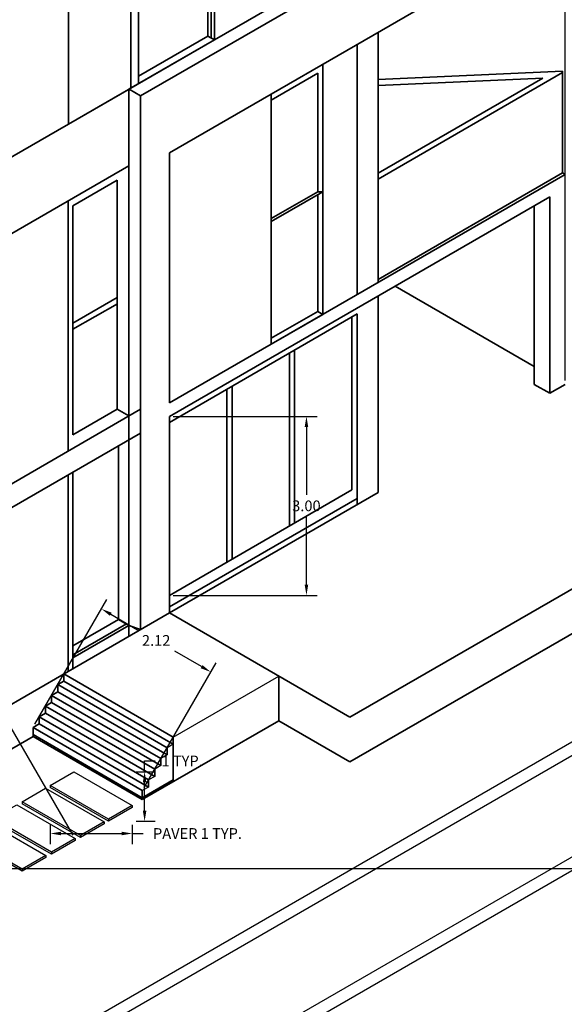
# Model space of a CAD drawing. Units: metres. Extents: x 12735 to 25554, y 20954 to 41989.
# Tile 13 of 15: x 12764 to 12773, y 20964 to 20981. Entities that reach past the tile are written whole.
import ezdxf

# ---------------------------------------------------------------- set-up
doc = ezdxf.new("R2010")
doc.units = ezdxf.units.M
doc.layers.get('Defpoints').update_dxf_attribs({"lineweight": 13})
for name, color, linetype, lineweight in [('A-ANNO-DIMS', 2, 'Continuous', 18), ('A-ELEV', 7, 'Continuous', 35), ('A-FLOR-STRS', 3, 'Continuous', 25), ('C-SITE', 8, 'Continuous', 25)]:
    doc.layers.add(name, color=color, linetype=linetype, lineweight=lineweight)
doc.styles.get("Standard").update_dxf_attribs({"font": 'arial.ttf'})
doc.dimstyles.get("Standard").update_dxf_attribs({"dimtxt": 0.18, "dimasz": 0.18, "dimexe": 0.18, "dimexo": 0.0625, "dimgap": 0.09, "dimtad": 0, "dimtih": 1, "dimtoh": 1, "dimdec": 4, "dimzin": 0, "dimdsep": 46, "dimtxsty": 'Standard', "dimcen": 0.09, "dimadec": 0, "dimazin": 0, "dimtfac": 1, "dimtdec": 4, "dimtofl": 0, "dimtmove": 0, "dimatfit": 3, "dimfxl": 1, "dimtolj": 1, "dimtzin": 0, "dimarcsym": 0})

# ---------------------------------------------------------------- blocks, each defined once
blk = doc.blocks.new('PAVER-STONE-A')
for p, q in [((0, 0.602), (0.397, 0.832)), ((0.397, 0.832), (1.377, 0.266)), ((0.98, 0.037), (0, 0.602)), ((0, 0.602), (0, 0.566)), ((0.98, 0), (0, 0.566)), ((1.377, 0.266), (0.98, 0.037)), ((1.377, 0.23), (0.98, 0)), ((1.377, 0.266), (1.377, 0.23)), ((0.98, 0.037), (0.98, 0))]:
    blk.add_line(p, q)
blk = doc.blocks.new('*D7')
at = {"layer": 'A-ANNO-DIMS', "color": 0, "lineweight": -2, "transparency": 16777216}
for p, q in [((12764.657, 20967.315), (12764.657, 20966.991)), ((12766.034, 20967.315), (12766.034, 20966.991)), ((12764.837, 20967.171), (12765.854, 20967.171)), ((12766.034, 20967.171), (12766.214, 20967.171))]:
    blk.add_line(p, q, dxfattribs=at)
at = {"layer": 'A-ANNO-DIMS', "color": 0, "transparency": 16777216}
for points in [[(12764.837, 20967.201), (12764.837, 20967.141), (12764.657, 20967.171)], [(12765.854, 20967.201), (12765.854, 20967.141), (12766.034, 20967.171)]]:
    blk.add_solid(points, dxfattribs=at)
at = {"layer": 'Defpoints', "color": 0, "transparency": 16777216}
for p in [(12764.657, 20967.377), (12766.034, 20967.377), (12766.034, 20967.171)]:
    blk.add_point(p, dxfattribs=at)
at = {"layer": 'A-ANNO-DIMS', "color": 0, "transparency": 16777216, "insert": (12767.129, 20967.171), "char_height": 0.18, "attachment_point": 5}
blk.add_mtext('\\A1;PAVER 1 TYP.', dxfattribs=at)
blk = doc.blocks.new('*D8')
at = {"layer": 'A-ANNO-DIMS', "color": 0, "lineweight": -2, "transparency": 16777216}
for p, q in [((12766.241, 20968.209), (12766.241, 20968.389)), ((12766.241, 20968.389), (12766.421, 20968.389)), ((12766.097, 20968.209), (12766.421, 20968.209)), ((12766.241, 20967.557), (12766.241, 20968.029)), ((12766.097, 20967.377), (12766.421, 20967.377))]:
    blk.add_line(p, q, dxfattribs=at)
at = {"layer": 'A-ANNO-DIMS', "color": 0, "transparency": 16777216}
for points in [[(12766.211, 20968.029), (12766.271, 20968.029), (12766.241, 20968.209)], [(12766.211, 20967.557), (12766.271, 20967.557), (12766.241, 20967.377)]]:
    blk.add_solid(points, dxfattribs=at)
at = {"layer": 'Defpoints', "color": 0, "transparency": 16777216}
for p in [(12766.034, 20968.209), (12766.241, 20968.209), (12766.034, 20967.377)]:
    blk.add_point(p, dxfattribs=at)
at = {"layer": 'A-ANNO-DIMS', "color": 0, "transparency": 16777216, "insert": (12766.871, 20968.389), "char_height": 0.18, "attachment_point": 5}
blk.add_mtext('\\A1;1 TYP.', dxfattribs=at)
blk = doc.blocks.new('*D9')
at = {"layer": 'A-ANNO-DIMS', "color": 0, "lineweight": -2, "transparency": 16777216}
for p, q in [((12781.004, 20970.87), (12781.004, 20953.893)), ((12737.843, 20966.671), (12737.843, 20953.893)), ((12738.023, 20954.073), (12759.026, 20954.073)), ((12780.824, 20954.073), (12759.821, 20954.073))]:
    blk.add_line(p, q, dxfattribs=at)
at = {"layer": 'A-ANNO-DIMS', "color": 0, "transparency": 16777216}
for points in [[(12738.023, 20954.103), (12738.023, 20954.043), (12737.843, 20954.073)], [(12780.824, 20954.103), (12780.824, 20954.043), (12781.004, 20954.073)]]:
    blk.add_solid(points, dxfattribs=at)
at = {"layer": 'Defpoints', "color": 0, "transparency": 16777216}
for p in [(12781.004, 20970.933), (12737.843, 20966.733), (12781.004, 20954.073)]:
    blk.add_point(p, dxfattribs=at)
at = {"layer": 'A-ANNO-DIMS', "color": 0, "transparency": 16777216, "insert": (12759.423, 20954.073), "char_height": 0.18, "attachment_point": 5}
blk.add_mtext('\\A1;43.16', dxfattribs=at)
blk = doc.blocks.new('*D10')
at = {"layer": 'A-ANNO-DIMS', "color": 0, "lineweight": -2, "transparency": 16777216}
for p, q in [((12766.645, 20994.825), (12783.484, 20994.825)), ((12783.304, 20994.645), (12783.304, 20975.781)), ((12783.304, 20956.553), (12783.304, 20975.417)), ((12755.849, 20956.373), (12783.484, 20956.373))]:
    blk.add_line(p, q, dxfattribs=at)
at = {"layer": 'A-ANNO-DIMS', "color": 0, "transparency": 16777216}
for points in [[(12783.274, 20994.645), (12783.334, 20994.645), (12783.304, 20994.825)], [(12783.274, 20956.553), (12783.334, 20956.553), (12783.304, 20956.373)]]:
    blk.add_solid(points, dxfattribs=at)
at = {"layer": 'Defpoints', "color": 0, "transparency": 16777216}
for p in [(12766.582, 20994.825), (12783.304, 20994.825), (12755.787, 20956.373)]:
    blk.add_point(p, dxfattribs=at)
at = {"layer": 'A-ANNO-DIMS', "color": 0, "transparency": 16777216, "insert": (12783.304, 20975.599), "char_height": 0.18, "attachment_point": 5}
blk.add_mtext('\\A1;38.45', dxfattribs=at)
blk = doc.blocks.new('*D12')
at = {"layer": 'A-ANNO-DIMS', "color": 0, "lineweight": -2, "transparency": 16777216}
for p, q in [((12781.035, 20970.878), (12782.244, 20968.785)), ((12781.998, 20968.851), (12769.861, 20961.843)), ((12757.093, 20954.472), (12769.23, 20961.479)), ((12755.818, 20956.319), (12757.027, 20954.226))]:
    blk.add_line(p, q, dxfattribs=at)
at = {"layer": 'A-ANNO-DIMS', "color": 0, "transparency": 16777216}
for points in [[(12781.983, 20968.877), (12782.013, 20968.825), (12782.154, 20968.941)], [(12757.078, 20954.497), (12757.108, 20954.446), (12756.937, 20954.382)]]:
    blk.add_solid(points, dxfattribs=at)
at = {"layer": 'Defpoints', "color": 0, "transparency": 16777216}
for p in [(12781.004, 20970.933), (12755.787, 20956.373), (12756.937, 20954.382)]:
    blk.add_point(p, dxfattribs=at)
at = {"layer": 'A-ANNO-DIMS', "color": 0, "transparency": 16777216, "insert": (12769.545, 20961.661), "char_height": 0.18, "attachment_point": 5}
blk.add_mtext('\\A1;29.12', dxfattribs=at)
blk = doc.blocks.new('*D14')
at = {"layer": 'A-ANNO-DIMS', "color": 0, "lineweight": -2, "transparency": 16777216}
for p, q in [((12766.7, 20994.856), (12783.484, 20994.856)), ((12783.304, 20994.676), (12783.304, 20980.902)), ((12783.304, 20966.764), (12783.304, 20980.538)), ((12760.589, 20966.584), (12783.484, 20966.584))]:
    blk.add_line(p, q, dxfattribs=at)
at = {"layer": 'A-ANNO-DIMS', "color": 0, "transparency": 16777216}
for points in [[(12783.274, 20994.676), (12783.334, 20994.676), (12783.304, 20994.856)], [(12783.274, 20966.764), (12783.334, 20966.764), (12783.304, 20966.584)]]:
    blk.add_solid(points, dxfattribs=at)
at = {"layer": 'Defpoints', "color": 0, "transparency": 16777216}
for p in [(12766.637, 20994.856), (12783.304, 20994.856), (12760.527, 20966.584)]:
    blk.add_point(p, dxfattribs=at)
at = {"layer": 'A-ANNO-DIMS', "color": 0, "transparency": 16777216, "insert": (12783.304, 20980.72), "char_height": 0.18, "attachment_point": 5}
blk.add_mtext('\\A1;28.273', dxfattribs=at)
blk = doc.blocks.new('*D19')
at = {"layer": 'A-ANNO-DIMS', "color": 0, "lineweight": -2, "transparency": 16777216}
for p, q in [((12747.33, 20976.079), (12747.33, 20997.336)), ((12773.306, 20974.774), (12773.306, 20997.336)), ((12747.51, 20997.156), (12759.853, 20997.156)), ((12773.126, 20997.156), (12760.783, 20997.156))]:
    blk.add_line(p, q, dxfattribs=at)
at = {"layer": 'A-ANNO-DIMS', "color": 0, "transparency": 16777216}
for points in [[(12747.51, 20997.186), (12747.51, 20997.126), (12747.33, 20997.156)], [(12773.126, 20997.186), (12773.126, 20997.126), (12773.306, 20997.156)]]:
    blk.add_solid(points, dxfattribs=at)
at = {"layer": 'Defpoints', "color": 0, "transparency": 16777216}
for p in [(12773.306, 20997.156), (12747.33, 20976.016), (12773.306, 20974.711)]:
    blk.add_point(p, dxfattribs=at)
at = {"layer": 'A-ANNO-DIMS', "color": 0, "transparency": 16777216, "insert": (12760.318, 20997.156), "char_height": 0.18, "attachment_point": 5}
blk.add_mtext('\\A1;25.976', dxfattribs=at)
blk = doc.blocks.new('*D25')
at = {"layer": 'A-ANNO-DIMS', "color": 0, "lineweight": -2, "transparency": 16777216}
for p, q in [((12764.398, 20969.005), (12765.607, 20971.098)), ((12765.673, 20970.852), (12766.122, 20970.593)), ((12767.197, 20969.972), (12766.747, 20970.232)), ((12766.234, 20967.945), (12767.443, 20970.038))]:
    blk.add_line(p, q, dxfattribs=at)
at = {"layer": 'A-ANNO-DIMS', "color": 0, "transparency": 16777216}
for points in [[(12765.688, 20970.878), (12765.658, 20970.826), (12765.517, 20970.942)], [(12767.212, 20969.998), (12767.182, 20969.946), (12767.353, 20969.882)]]:
    blk.add_solid(points, dxfattribs=at)
at = {"layer": 'Defpoints', "color": 0, "transparency": 16777216}
for p in [(12767.353, 20969.882), (12764.367, 20968.95), (12766.203, 20967.89)]:
    blk.add_point(p, dxfattribs=at)
at = {"layer": 'A-ANNO-DIMS', "color": 0, "transparency": 16777216, "insert": (12766.435, 20970.412), "char_height": 0.18, "attachment_point": 5}
blk.add_mtext('\\A1;2.12', dxfattribs=at)
blk = doc.blocks.new('*D27')
at = {"layer": 'A-ANNO-DIMS', "color": 0, "lineweight": -2, "transparency": 16777216}
for p, q in [((12765.041, 20967.142), (12763.833, 20969.236)), ((12763.767, 20968.99), (12762.465, 20968.238)), ((12760.533, 20967.123), (12761.835, 20967.874)), ((12761.496, 20965.095), (12760.287, 20967.189))]:
    blk.add_line(p, q, dxfattribs=at)
at = {"layer": 'A-ANNO-DIMS', "color": 0, "transparency": 16777216}
for points in [[(12763.752, 20969.016), (12763.782, 20968.964), (12763.923, 20969.08)], [(12760.518, 20967.149), (12760.548, 20967.097), (12760.377, 20967.033)]]:
    blk.add_solid(points, dxfattribs=at)
at = {"layer": 'Defpoints', "color": 0, "transparency": 16777216}
for p in [(12763.923, 20969.08), (12765.073, 20967.088), (12761.527, 20965.041)]:
    blk.add_point(p, dxfattribs=at)
at = {"layer": 'A-ANNO-DIMS', "color": 0, "transparency": 16777216, "insert": (12762.15, 20968.056), "char_height": 0.18, "attachment_point": 5}
blk.add_mtext('\\A1;4.094', dxfattribs=at)
blk = doc.blocks.new('*D28')
at = {"layer": 'A-ANNO-DIMS', "color": 0, "lineweight": -2, "transparency": 16777216}
for p, q in [((12766.721, 20974.174), (12769.139, 20974.174)), ((12768.959, 20973.994), (12768.959, 20972.854)), ((12768.959, 20971.349), (12768.959, 20972.49)), ((12766.721, 20971.169), (12769.139, 20971.169))]:
    blk.add_line(p, q, dxfattribs=at)
at = {"layer": 'A-ANNO-DIMS', "color": 0, "transparency": 16777216}
for points in [[(12768.929, 20973.994), (12768.989, 20973.994), (12768.959, 20974.174)], [(12768.929, 20971.349), (12768.989, 20971.349), (12768.959, 20971.169)]]:
    blk.add_solid(points, dxfattribs=at)
at = {"layer": 'Defpoints', "color": 0, "transparency": 16777216}
for p in [(12766.659, 20974.174), (12766.659, 20971.169), (12768.959, 20971.169)]:
    blk.add_point(p, dxfattribs=at)
at = {"layer": 'A-ANNO-DIMS', "color": 0, "transparency": 16777216, "insert": (12768.959, 20972.672), "char_height": 0.18, "attachment_point": 5}
blk.add_mtext('\\A1;3.00', dxfattribs=at)

msp = doc.modelspace()

# ---------------------------------------------------------------- linework, layer by layer
at = {"layer": 'A-ELEV'}
for p, q in [((12765.9783, 20979.6678), (12772.884, 20983.6548)), ((12766.174, 20979.5548), (12773.2754, 20983.6548)), ((12767.3582, 20982.9804), (12767.3582, 20980.5265)), ((12767.4127, 20983.0118), (12767.4127, 20980.495)), ((12767.3037, 20982.9175), (12767.3037, 20980.5579)), ((12766.6589, 20978.5998), (12773.2754, 20982.4199)), ((12766.0102, 20982.1706), (12766.0102, 20979.6853)), ((12766.1361, 20982.2434), (12766.1361, 20979.758)), ((12764.963, 20981.5975), (12764.963, 20979.0807)), ((12767.4127, 20980.495), (12764.963, 20979.0807)), ((12767.3037, 20980.5579), (12766.1361, 20979.8838)), ((12767.4127, 20980.495), (12767.3037, 20980.5579)), ((12770.1643, 20976.4237), (12770.1643, 20980.6237)), ((12769.8103, 20976.2193), (12769.8103, 20980.4193)), ((12769.2346, 20980.0869), (12769.2346, 20975.8869)), ((12768.365, 20979.4848), (12769.148, 20979.9369)), ((12769.148, 20979.9369), (12769.148, 20977.9457)), ((12770.1643, 20979.8287), (12773.2624, 20979.9687)), ((12770.1643, 20978.157), (12773.2624, 20979.9457)), ((12770.1643, 20978.257), (12772.9299, 20979.8537)), ((12770.1643, 20979.7287), (12772.9299, 20979.8537)), ((12773.2624, 20978.2623), (12773.2624, 20979.9687)), ((12765.9791, 20979.6673), (12760.2287, 20976.3473)), ((12765.9783, 20974.1809), (12765.9783, 20979.6678)), ((12766.174, 20979.5548), (12765.9791, 20979.6673)), ((12766.174, 20970.5939), (12766.174, 20979.5548)), ((12768.365, 20979.5848), (12768.365, 20975.3848)), ((12766.6589, 20974.3998), (12766.6589, 20978.5998)), ((12761.5277, 20975.8113), (12765.9783, 20978.3809)), ((12766.6589, 20974.3998), (12773.3057, 20978.2373)), ((12770.1643, 20976.4737), (12773.2624, 20978.2623)), ((12773.3057, 20978.2373), (12773.2624, 20978.2623)), ((12765.037, 20977.7077), (12765.7826, 20978.1381)), ((12765.7826, 20974.2939), (12765.7826, 20978.1381)), ((12766.6589, 20974.1738), (12773.0459, 20977.8613)), ((12768.365, 20977.4936), (12769.148, 20977.9457)), ((12768.365, 20977.4436), (12769.2346, 20977.9457)), ((12769.2346, 20977.9457), (12769.148, 20977.9457)), ((12769.148, 20977.8957), (12769.148, 20975.9369)), ((12773.0459, 20977.8613), (12773.0459, 20974.5613)), ((12764.959, 20973.5924), (12764.959, 20977.7924)), ((12765.037, 20973.8634), (12765.037, 20977.7077)), ((12772.7861, 20977.7113), (12772.7861, 20974.7113)), ((12772.7861, 20975.0113), (12770.4478, 20976.3613)), ((12770.1643, 20976.1977), (12770.1643, 20972.8977)), ((12765.037, 20975.7374), (12765.7826, 20976.1679)), ((12765.0377, 20975.6355), (12765.7833, 20976.066)), ((12766.6589, 20974.0738), (12769.8103, 20975.8933)), ((12768.365, 20975.4848), (12769.148, 20975.9369)), ((12768.365, 20975.3848), (12769.2346, 20975.8869)), ((12769.2346, 20975.8869), (12769.148, 20975.9369)), ((12769.8103, 20972.6933), (12769.8103, 20975.8933)), ((12769.7237, 20972.9388), (12769.7237, 20975.8433)), ((12768.6732, 20975.2368), (12768.6732, 20972.3323)), ((12768.7598, 20975.2868), (12768.7598, 20972.3823)), ((12772.7861, 20974.7113), (12773.0459, 20974.5613)), ((12773.0459, 20974.5613), (12773.3057, 20974.7113)), ((12767.6228, 20974.6303), (12767.6228, 20971.7259)), ((12767.7094, 20974.6803), (12767.7094, 20971.7759)), ((12760.2287, 20970.8613), (12766.174, 20974.2939)), ((12765.037, 20973.8634), (12765.7826, 20974.2939)), ((12765.9783, 20974.1809), (12765.7826, 20974.2939)), ((12765.9783, 20970.4809), (12765.9783, 20974.1809)), ((12766.6589, 20970.8738), (12766.6589, 20974.1738)), ((12760.2287, 20970.4613), (12766.174, 20973.8939)), ((12765.8027, 20970.7648), (12765.8027, 20973.6795)), ((12765.037, 20969.9374), (12765.037, 20973.2374)), ((12764.959, 20969.8924), (12764.959, 20973.1924)), ((12769.7237, 20972.9388), (12766.6589, 20971.1694)), ((12770.1643, 20972.8977), (12766.6589, 20970.8738)), ((12776.3368, 20972.9613), (12769.69, 20969.1238)), ((12769.8103, 20972.7933), (12766.6589, 20970.9738)), ((12776.3368, 20972.2113), (12769.69, 20968.3738)), ((12764.959, 20969.8924), (12766.6589, 20970.8738)), ((12765.037, 20970.3227), (12765.8027, 20970.7648)), ((12765.9783, 20970.6634), (12765.8027, 20970.7648)), ((12766.6589, 20970.8738), (12769.69, 20969.1238)), ((12765.037, 20970.17), (12765.935, 20970.6884)), ((12765.037, 20970.12), (12765.9783, 20970.6634)), ((12766.174, 20970.5939), (12765.9783, 20970.6634)), ((12760.5269, 20967.3335), (12764.959, 20969.8924)), ((12764.8863, 20969.8504), (12766.7223, 20968.7904)), ((12764.8863, 20969.8504), (12764.8863, 20969.7304)), ((12768.4949, 20969.8139), (12768.4949, 20969.0639)), ((12764.8863, 20969.7304), (12764.7824, 20969.6704)), ((12766.6184, 20968.6104), (12764.7824, 20969.6704)), ((12764.7824, 20969.6704), (12764.7824, 20969.5504)), ((12764.8863, 20969.7304), (12766.7223, 20968.6704)), ((12764.7824, 20969.5504), (12764.6785, 20969.4904)), ((12766.5144, 20968.4304), (12764.6785, 20969.4904)), ((12764.6785, 20969.4904), (12764.6785, 20969.3704)), ((12766.6184, 20968.4904), (12764.7824, 20969.5504)), ((12764.6785, 20969.3704), (12764.5746, 20969.3104)), ((12766.4105, 20968.2504), (12764.5746, 20969.3104)), ((12764.5746, 20969.3104), (12764.5746, 20969.1904)), ((12766.5144, 20968.3104), (12764.6785, 20969.3704)), ((12766.5144, 20968.3104), (12764.6785, 20969.3704)), ((12764.5746, 20969.1904), (12764.4706, 20969.1304)), ((12766.3066, 20968.0704), (12764.4706, 20969.1304)), ((12764.4706, 20969.1304), (12764.4706, 20969.0104)), ((12766.4105, 20968.1304), (12764.5746, 20969.1904)), ((12766.4105, 20968.1304), (12764.5746, 20969.1904)), ((12764.4706, 20969.0104), (12764.3667, 20968.9504)), ((12766.2027, 20967.8904), (12764.3667, 20968.9504)), ((12764.3667, 20968.9504), (12764.3667, 20968.8004)), ((12766.3066, 20967.9504), (12764.4706, 20969.0104)), ((12766.3066, 20967.9504), (12764.4706, 20969.0104)), ((12766.3066, 20967.9504), (12764.4706, 20969.0104)), ((12768.4949, 20969.0639), (12766.2027, 20967.7404)), ((12768.4949, 20969.0639), (12769.69, 20968.3738)), ((12760.5269, 20966.5835), (12764.3667, 20968.8004)), ((12766.2027, 20967.7704), (12764.3667, 20968.8304)), ((12766.2027, 20967.7404), (12764.3667, 20968.8004)), ((12766.7223, 20968.7904), (12766.7223, 20968.0404)), ((12766.6184, 20968.6104), (12766.6184, 20968.4904)), ((12766.5144, 20968.4304), (12766.5144, 20968.3104)), ((12766.4105, 20968.2504), (12766.4105, 20968.1304)), ((12766.2027, 20967.7704), (12766.7223, 20968.0704)), ((12766.3066, 20968.0704), (12766.3066, 20967.9504)), ((12766.2027, 20967.8904), (12766.2027, 20967.7404))]:
    msp.add_line(p, q, dxfattribs=at)
at = {"layer": 'A-FLOR-STRS'}
for p, q in [((12766.7223, 20968.7904), (12768.4949, 20969.8139)), ((12766.7223, 20968.6704), (12766.6184, 20968.6104)), ((12766.6184, 20968.4904), (12766.5144, 20968.4304)), ((12766.5144, 20968.3104), (12766.4105, 20968.2504)), ((12766.4105, 20968.1304), (12766.3066, 20968.0704)), ((12766.3066, 20967.9504), (12766.2027, 20967.8904))]:
    msp.add_line(p, q, dxfattribs=at)
at = {"layer": 'C-SITE'}
for p, q in [((12780.6127, 20972.8586), (12757.9519, 20959.7754)), ((12781.0041, 20972.8586), (12757.9519, 20959.5494)), ((12781.0041, 20971.1586), (12755.7869, 20956.5994)), ((12755.7869, 20956.3734), (12781.0041, 20970.9326))]:
    msp.add_line(p, q, dxfattribs=at)
at = {"layer": 'Defpoints'}
for p in [(12768.7598, 20975.2868), (12767.7094, 20974.6803)]:
    msp.add_point(p, dxfattribs=at)

# ---------------------------------------------------------------- block references
at = {"layer": 'C-SITE'}
for p in [(12764.657, 20967.377), (12764.182, 20967.1028), (12763.6953, 20966.8218), (12763.2033, 20966.5377)]:
    msp.add_blockref('PAVER-STONE-A', p, dxfattribs=at)

# ---------------------------------------------------------------- dimensions: what is measured, and where the dimension line sits
at = {"layer": 'A-ANNO-DIMS'}
for base, p1, p2, override, picture, middle in [((12773.3057, 20997.1564), (12747.3297, 20976.0163), (12773.3057, 20974.7113), {"dimdec": 3, "dimlfac": 1, "dimrnd": 0, "dimzin": 0, "dimdsep": 46, "dimlunit": 2}, '*D19', (12760.3177, 20997.1564)), ((12781.0041, 20954.0734), (12737.8426, 20966.7335), (12781.0041, 20970.9326), {"dimdec": 2, "dimlfac": 1, "dimrnd": 0, "dimzin": 0, "dimdsep": 46, "dimlunit": 2}, '*D9', (12759.4234, 20954.0734))]:
    dim = msp.add_linear_dim(base=base, p1=p1, p2=p2, dimstyle='Standard', override=override, dxfattribs=at)
    dim.commit()
    dim.dimension.update_dxf_attribs({"geometry": picture, "text_midpoint": middle})
for base, p1, p2, angle, override, picture, middle in [((12783.3041, 20994.8247), (12755.7869, 20956.3734), (12766.582, 20994.8247), 90, {"dimdec": 2, "dimlfac": 1, "dimrnd": 0, "dimzin": 0, "dimdsep": 46, "dimlunit": 2}, '*D10', (12783.3041, 20975.599)), ((12783.3041, 20994.8564), (12760.5269, 20966.5835), (12766.637, 20994.8564), 90, {"dimdec": 3, "dimlfac": 1, "dimrnd": 0, "dimzin": 0, "dimdsep": 46, "dimlunit": 2}, '*D14', (12783.3041, 20980.72)), ((12768.9589, 20971.1694), (12766.6589, 20974.1738), (12766.6589, 20971.1694), 270, {"dimdec": 2, "dimlfac": 1, "dimrnd": 0, "dimzin": 0, "dimdsep": 46, "dimlunit": 2}, '*D28', (12768.9589, 20972.6716)), ((12767.3527, 20969.8823), (12764.3667, 20968.9504), (12766.2027, 20967.8904), 330, {"dimdec": 2, "dimlfac": 1, "dimrnd": 0, "dimzin": 0, "dimdsep": 46, "dimlunit": 2}, '*D25', (12766.4347, 20970.4123)), ((12756.9369, 20954.3815), (12781.0041, 20970.9326), (12755.7869, 20956.3734), 210, {"dimdec": 2, "dimlfac": 1, "dimrnd": 0, "dimzin": 0, "dimdsep": 46, "dimlunit": 2}, '*D12', (12769.5455, 20961.6611)), ((12763.9225, 20969.0798), (12761.5271, 20965.041), (12765.0725, 20967.0879), 30, {"dimdec": 3, "dimlfac": 1, "dimrnd": 0, "dimzin": 0, "dimdsep": 46, "dimlunit": 2}, '*D27', (12762.1498, 20968.0563))]:
    dim = msp.add_linear_dim(base=base, p1=p1, p2=p2, angle=angle, dimstyle='Standard', override=override, dxfattribs=at)
    dim.commit()
    dim.dimension.update_dxf_attribs({"geometry": picture, "text_midpoint": middle})
dim = msp.add_linear_dim(base=(12766.2408, 20968.2089), p1=(12766.0342, 20967.3775), p2=(12766.0342, 20968.2089), angle=90, text='<> TYP.', dimstyle='Standard', override={"dimdec": 0, "dimlfac": 1, "dimrnd": 0, "dimzin": 0, "dimdsep": 46, "dimlunit": 2}, dxfattribs=at)
dim.commit()
dim.dimension.update_dxf_attribs({"geometry": '*D8', "text_midpoint": (12766.8705, 20968.3889)})
dim = msp.add_linear_dim(base=(12766.0342, 20967.1709), p1=(12764.6571, 20967.3775), p2=(12766.0342, 20967.3775), text='PAVER <> TYP.', dimstyle='Standard', override={"dimdec": 0, "dimlfac": 1, "dimrnd": 0, "dimzin": 0, "dimdsep": 46, "dimlunit": 2}, dxfattribs=at)
dim.commit()
dim.dimension.update_dxf_attribs({"geometry": '*D7', "text_midpoint": (12767.1291, 20967.1709)})

doc.saveas('drawing.dxf')
